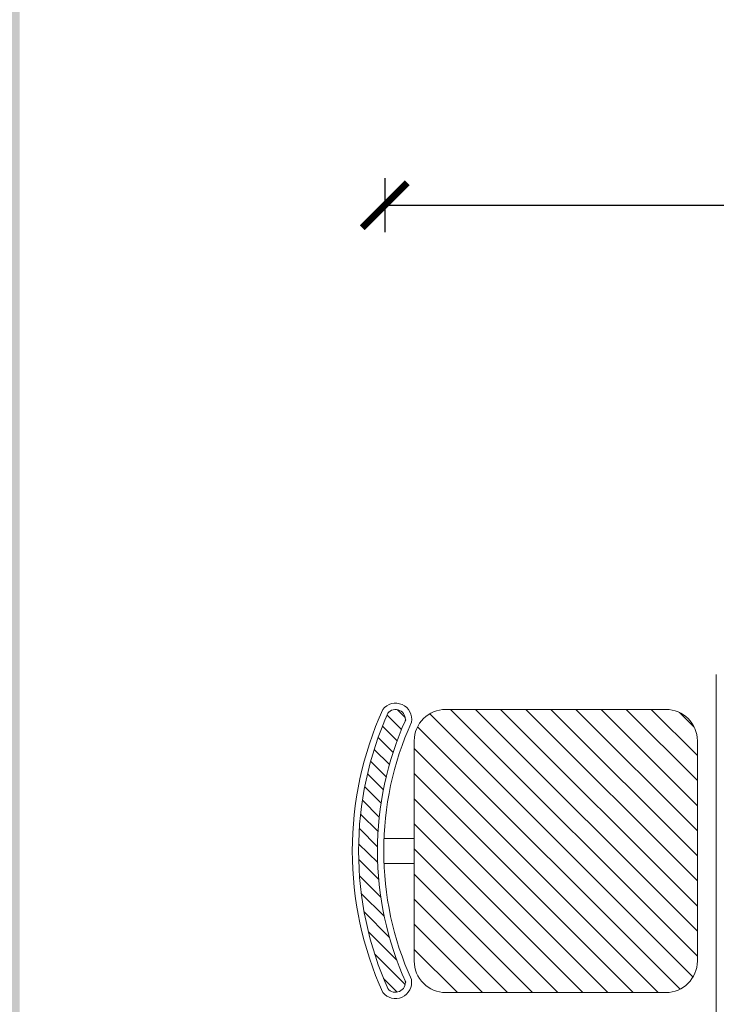
# Model space of a CAD drawing. Units: inches. Extents: x 375 to 1122, y 27 to 1069.
# Tile 115 of 155: x 667 to 705, y 887 to 941. Entities that reach past the tile are written whole.
import ezdxf

# ---------------------------------------------------------------- set-up
doc = ezdxf.new("R2010")
doc.units = ezdxf.units.IN
for name, color, linetype, lineweight in [('A-ANNO-DIMS', 2, 'Continuous', 18), ('A-WALL-PATT', 252, 'Continuous', 13), ('Furniture', 30, 'Continuous', 18)]:
    doc.layers.add(name, color=color, linetype=linetype, lineweight=lineweight)
doc.styles.get("Standard").update_dxf_attribs({"font": 'arial.ttf'})
doc.dimstyles.new('ISO-25', dxfattribs={"dimtxt": 12, "dimasz": 2.5, "dimexe": 1.5, "dimexo": 1.5, "dimtad": 1, "dimdec": 1, "dimlunit": 3, "dimtxsty": 'Standard', "dimblk": 'ARCHTICK', "dimcen": 2.5, "dimadec": 0, "dimazin": 0, "dimtfac": 1, "dimtdec": 1, "dimtmove": 0, "dimatfit": 3, "dimfxl": 1.5, "dimfxlon": 1, "dimarcsym": 0})

# ---------------------------------------------------------------- blocks, each defined once
blk = doc.blocks.new('A$C403C54AD')
for p, q in [((0.8357, 0.5048, -0.0006), (1.9992, 0.5048, -0.0006)), ((1.2329, 0.4785, -0.0006), (0.9275, 0.4785, -0.0006)), ((0.8839, 0.4349, -0.0006), (0.8839, 0.304, -0.0006)), ((1.2765, 0.1295, -0.0006), (1.2765, 0.4349, -0.0006)), ((0.8839, 0.304, -0.0006), (0.8839, 0.1295, -0.0006)), ((0.9275, 0.0859, -0.0006), (1.2329, 0.0859, -0.0006)), ((1.0628, 0.0859, -0.0006), (1.0628, 0.0436, -0.0006)), ((1.0977, 0.0859, -0.0006), (1.0977, 0.0436, -0.0006))]:
    blk.add_line(p, q)
at = {"ltscale": 0.05}
for p, q in [((1.2263, 0.4785, -0.0006), (0.8839, 0.1361, -0.0006)), ((1.1915, 0.4785, -0.0006), (0.8839, 0.1709, -0.0006)), ((1.1567, 0.4785, -0.0006), (0.8839, 0.2057, -0.0006)), ((1.1218, 0.4785, -0.0006), (0.8839, 0.2406, -0.0006)), ((1.087, 0.4785, -0.0006), (0.8839, 0.2754, -0.0006)), ((1.0522, 0.4785, -0.0006), (0.8839, 0.3102, -0.0006)), ((1.0174, 0.4785, -0.0006), (0.8839, 0.3451, -0.0006)), ((0.9825, 0.4785, -0.0006), (0.8839, 0.3799, -0.0006)), ((0.9477, 0.4785, -0.0006), (0.8839, 0.4147, -0.0006)), ((0.9085, 0.4742, -0.0006), (0.8882, 0.4539, -0.0006)), ((1.2551, 0.4725, -0.0006), (0.8899, 0.1073, -0.0006)), ((1.2719, 0.4545, -0.0006), (0.9079, 0.0905, -0.0006)), ((1.2765, 0.4243, -0.0006), (0.9381, 0.0859, -0.0006)), ((1.2765, 0.3895, -0.0006), (0.973, 0.0859, -0.0006)), ((1.2765, 0.3546, -0.0006), (1.0078, 0.0859, -0.0006)), ((1.2765, 0.3198, -0.0006), (1.0426, 0.0859, -0.0006)), ((1.2765, 0.285, -0.0006), (1.0774, 0.0859, -0.0006)), ((1.2765, 0.2501, -0.0006), (1.1123, 0.0859, -0.0006)), ((1.2765, 0.2153, -0.0006), (1.1471, 0.0859, -0.0006)), ((1.2765, 0.1805, -0.0006), (1.1819, 0.0859, -0.0006)), ((1.2765, 0.1457, -0.0006), (1.2168, 0.0859, -0.0006)), ((0.8952, 0.0734, -0.0006), (0.8843, 0.0625, -0.0006)), ((1.2652, 0.0733, -0.0006), (1.2228, 0.0309, -0.0006)), ((0.9118, 0.0682, -0.0006), (0.8918, 0.0483, -0.0006)), ((0.9274, 0.0621, -0.0006), (0.9072, 0.0418, -0.0006)), ((0.9436, 0.0565, -0.0006), (0.923, 0.0359, -0.0006)), ((1.2317, 0.0616, -0.0006), (1.1924, 0.0224, -0.0006)), ((1.276, 0.0624, -0.0006), (1.2569, 0.0433, -0.0006)), ((0.9603, 0.0515, -0.0006), (0.9393, 0.0304, -0.0006)), ((0.9776, 0.047, -0.0006), (0.9561, 0.0255, -0.0006)), ((0.9955, 0.0431, -0.0006), (0.9734, 0.021, -0.0006)), ((1.1708, 0.0443, -0.0006), (1.139, 0.0124, -0.0006)), ((1.1996, 0.0513, -0.0006), (1.1647, 0.0164, -0.0006)), ((1.014, 0.0399, -0.0006), (0.9914, 0.0172, -0.0006)), ((1.0333, 0.0374, -0.0006), (1.0099, 0.014, -0.0006)), ((1.0534, 0.0357, -0.0006), (1.0292, 0.0115, -0.0006)), ((1.0744, 0.0349, -0.0006), (1.0492, 0.0098, -0.0006)), ((1.0964, 0.0352, -0.0006), (1.0701, 0.0088, -0.0006)), ((1.1197, 0.0367, -0.0006), (1.0919, 0.0089, -0.0006)), ((1.1443, 0.0396, -0.0006), (1.1148, 0.01, -0.0006))]:
    blk.add_line(p, q, dxfattribs=at)
for centre, radius, start, end in [((0.9275, 0.4349, -0.0006), 0.0436, 90, 180), ((1.2329, 0.4349, -0.0006), 0.0436, 0, 90), ((0.9275, 0.1295, -0.0006), 0.0436, 180, 270), ((1.2329, 0.1295, -0.0006), 0.0436, 270, 0), ((0.8978, 0.0599, -0.0006), 0.0225, 79.7658, 231.6694), ((1.0802, 0.4774, -0.0006), 0.4338, 245.7176, 294.2824), ((1.2624, 0.0598, -0.0006), 0.0225, 308.8964, 99.6684), ((0.8978, 0.0599, -0.0006), 0.0138, 79.7658, 231.6694), ((1.0802, 0.4774, -0.0006), 0.4425, 245.7176, 294.2824), ((1.2624, 0.0598, -0.0006), 0.0138, 308.8964, 99.6684), ((1.0802, 0.4774, -0.0006), 0.4774, 245.7176, 294.2824), ((1.0802, 0.4774, -0.0006), 0.4687, 245.7176, 294.2824)]:
    blk.add_arc(centre, radius, start, end)
blk = doc.blocks.new('_ArchTick')
at = {"color": 0, "linetype": 'ByBlock', "const_width": 0.15}
blk.add_lwpolyline([(-0.5, -0.5), (0.5, 0.5)], dxfattribs=at)
blk = doc.blocks.new('*D58')
at = {"layer": 'A-ANNO-DIMS', "color": 0, "lineweight": -2, "transparency": 16777216}
for p, q in [((656.912, 835.528), (656.912, 940.287)), ((655.412, 835.528), (658.412, 835.528)), ((656.912, 750.836), (656.912, 835.528)), ((655.412, 750.836), (658.412, 750.836))]:
    blk.add_line(p, q, dxfattribs=at)
at = {"layer": 'Defpoints', "color": 0, "transparency": 16777216}
for p in [(638.071, 835.528), (656.912, 835.528), (638.071, 750.836)]:
    blk.add_point(p, dxfattribs=at)
at = {"layer": 'A-ANNO-DIMS', "color": 0, "lineweight": -2, "transparency": 16777216, "xscale": 2.5, "yscale": 2.5, "zscale": 2.5}
for p, rotation in [((656.912, 835.528), 90), ((656.912, 750.836), 270)]:
    blk.add_blockref('_ArchTick', p, dxfattribs=dict(at, rotation=rotation))
at = {"layer": 'A-ANNO-DIMS', "color": 0, "transparency": 16777216, "insert": (650.082, 889.157), "char_height": 12, "attachment_point": 5, "rotation": 90}
blk.add_mtext('7\'-0 1/2" TYP.', dxfattribs=at)
blk = doc.blocks.new('*D73')
at = {"layer": 'A-ANNO-DIMS', "color": 0, "lineweight": -2, "transparency": 16777216}
for p, q in [((686.757, 932.428), (686.757, 929.428)), ((770.757, 932.428), (770.757, 929.428)), ((686.757, 930.928), (770.757, 930.928)), ((770.757, 930.928), (987.61, 930.928))]:
    blk.add_line(p, q, dxfattribs=at)
at = {"layer": 'Defpoints', "color": 0, "transparency": 16777216}
for p in [(686.757, 943.528), (770.757, 943.528), (770.757, 930.928)]:
    blk.add_point(p, dxfattribs=at)
at = {"layer": 'A-ANNO-DIMS', "color": 0, "lineweight": -2, "transparency": 16777216, "xscale": 2.5, "yscale": 2.5, "zscale": 2.5, "rotation": 180}
blk.add_blockref('_ArchTick', (686.757, 930.928), dxfattribs=at)
at = {"layer": 'A-ANNO-DIMS', "color": 0, "lineweight": -2, "transparency": 16777216, "xscale": 2.5, "yscale": 2.5, "zscale": 2.5}
blk.add_blockref('_ArchTick', (770.757, 930.928), dxfattribs=at)
at = {"layer": 'A-ANNO-DIMS', "color": 0, "transparency": 16777216, "insert": (880.433, 937.757), "char_height": 12, "attachment_point": 5}
blk.add_mtext('2-PANEL SLIDER 7\'-0" TYP.', dxfattribs=at)

msp = doc.modelspace()

# ---------------------------------------------------------------- hatches: boundary and pattern name
at = {"layer": 'A-WALL-PATT'}
h = msp.add_hatch(color=256, dxfattribs=at)
h.dxf.hatch_style = 1
h.paths.add_polyline_path([(962.007, 388.528), (989.007, 388.528), (989.007, 394.528), (962.007, 394.528), (932.007, 394.528), (932.007, 397.528), (923.007, 397.528), (923.007, 394.528), (842.007, 394.528), (842.007, 334.528), (839.507, 334.528), (839.507, 328.528), (854.007, 328.528), (854.007, 334.528), (848.007, 334.528), (848.007, 388.528), (953.007, 388.528), (953.007, 356.081), (962.007, 356.081), (962.007, 358.554), (989.007, 358.554), (989.007, 364.554), (962.007, 364.554)])
h.paths.add_polyline_path([(989.007, 502.528), (932.007, 502.528), (932.007, 583.528), (932.007, 593.528), (923.007, 593.528), (923.007, 583.528), (854.007, 583.528), (854.007, 556.528), (863.007, 556.528), (863.007, 574.528), (923.007, 574.528), (923.007, 502.528), (863.007, 502.528), (863.007, 520.528), (854.007, 520.528), (854.007, 502.528), (773.007, 502.528), (773.007, 493.528), (788.007, 493.528), (788.007, 402.028), (722.007, 402.028), (722.007, 373.528), (728.007, 373.528), (728.007, 396.028), (788.007, 396.028), (788.007, 373.528), (794.007, 373.528), (794.007, 430.528), (814.007, 430.528), (814.007, 436.528), (794.007, 436.528), (794.007, 493.528), (923.007, 493.528), (923.007, 487.528), (932.007, 487.528), (932.007, 493.528), (983.007, 493.528), (983.007, 473.528), (989.007, 473.528)])
h.paths.add_polyline_path([(797.007, 325.528), (805.007, 325.528), (805.007, 328.528), (807.507, 328.528), (807.507, 334.528), (791.007, 334.528), (791.007, 226.528), (770.757, 226.528), (770.757, 217.528), (791.007, 217.528), (791.007, 187.528), (855.007, 187.528), (855.007, 196.528), (797.007, 196.528)])
h.paths.add_polyline_path([(989.007, 238.528), (962.007, 238.528), (962.007, 256.424), (953.007, 256.424), (953.007, 229.528), (980.007, 229.528), (980.007, 196.528), (915.007, 196.528), (915.007, 187.528), (989.007, 187.528)])
h.paths.add_polyline_path([(962.007, 334.528), (884.007, 334.528), (884.007, 328.528), (918.007, 328.528), (918.007, 325.528), (932.007, 325.528), (932.007, 328.528), (953.007, 328.528), (953.007, 304.424), (962.007, 304.424)])
h.paths.add_polyline_path([(606.507, 283.528), (609.507, 283.528), (609.507, 289.528), (600.507, 289.528), (600.507, 196.528), (578.507, 196.528), (578.507, 187.528), (606.507, 187.528), (606.507, 196.528)])
h.paths.add_polyline_path([(666.507, 292.528), (660.507, 292.528), (660.507, 289.528), (633.507, 289.528), (633.507, 283.528), (660.507, 283.528), (660.507, 196.528), (628.007, 196.528), (628.007, 187.528), (630.534, 187.528), (630.534, 160.528), (636.534, 160.528), (636.534, 187.528), (660.507, 187.528), (660.507, 160.528), (666.507, 160.528), (666.507, 217.528), (686.757, 217.528), (686.757, 226.528), (666.507, 226.528)])
h.paths.add_polyline_path([(480.507, 256.424), (471.507, 256.424), (471.507, 238.528), (444.507, 238.528), (444.507, 187.528), (518.507, 187.528), (518.507, 196.528), (453.507, 196.528), (453.507, 229.528), (480.507, 229.528)])
h.paths.add_polyline_path([(480.507, 328.528), (652.507, 328.528), (652.507, 325.528), (660.507, 325.528), (660.507, 322.528), (666.507, 322.528), (666.507, 334.528), (507.507, 334.528), (507.507, 360.528), (498.507, 360.528), (498.507, 334.528), (471.507, 334.528), (471.507, 304.424), (480.507, 304.424)])
h.paths.add_polyline_path([(507.507, 484.528), (498.507, 484.528), (498.507, 444.528), (507.507, 444.528), (507.507, 454.528), (621.507, 454.528), (621.507, 460.528), (507.507, 460.528)])
h.paths.add_polyline_path([(672.507, 604.528), (683.257, 604.528), (683.257, 613.528), (669.507, 613.528), (669.507, 649.528), (663.507, 649.528), (663.507, 589.528), (507.507, 589.528), (507.507, 613.528), (498.507, 613.528), (498.507, 556.528), (507.507, 556.528), (507.507, 580.528), (663.507, 580.528), (663.507, 520.528), (669.507, 520.528), (669.507, 556.528), (683.257, 556.528), (683.257, 565.528), (672.507, 565.528)])
h.paths.add_polyline_path([(731.007, 667.528), (734.007, 667.528), (734.007, 676.528), (728.007, 676.528), (728.007, 715.528), (657.507, 715.528), (657.507, 709.528), (663.507, 709.528), (663.507, 673.528), (669.507, 673.528), (669.507, 709.528), (722.007, 709.528), (722.007, 613.528), (704.757, 613.528), (704.757, 604.528), (722.007, 604.528), (722.007, 565.528), (704.757, 565.528), (704.757, 556.528), (722.007, 556.528), (722.007, 502.528), (722.007, 460.528), (669.507, 460.528), (669.507, 496.528), (663.507, 496.528), (663.507, 460.528), (657.507, 460.528), (657.507, 454.528), (728.007, 454.528), (728.007, 493.528), (734.007, 493.528), (734.007, 502.528), (731.007, 502.528)])
h.paths.add_polyline_path([(986.007, 718.528), (959.007, 718.528), (959.007, 727.528), (950.007, 727.528), (950.007, 709.528), (977.007, 709.528), (977.007, 676.528), (794.007, 676.528), (794.007, 805.528), (802.007, 805.528), (802.007, 808.528), (804.507, 808.528), (804.507, 814.528), (788.007, 814.528), (788.007, 774.028), (728.007, 774.028), (728.007, 796.528), (722.007, 796.528), (722.007, 768.028), (788.007, 768.028), (788.007, 676.528), (773.007, 676.528), (773.007, 667.528), (923.007, 667.528), (923.007, 657.528), (932.007, 657.528), (932.007, 667.528), (986.007, 667.528)])
h.paths.add_polyline_path([(621.507, 715.528), (507.507, 715.528), (507.507, 733.528), (498.507, 733.528), (498.507, 715.528), (498.507, 685.528), (507.507, 685.528), (507.507, 709.528), (621.507, 709.528)])
h.paths.add_polyline_path([(666.507, 847.028), (660.507, 847.028), (660.507, 844.528), (652.507, 844.528), (652.507, 841.528), (480.507, 841.528), (480.507, 859.528), (471.507, 859.528), (471.507, 835.528), (498.507, 835.528), (498.507, 817.528), (507.507, 817.528), (507.507, 835.528), (666.507, 835.528)])
h.paths.add_polyline_path([(480.507, 940.528), (453.507, 940.528), (453.507, 973.528), (518.507, 973.528), (518.507, 982.528), (444.507, 982.528), (444.507, 931.528), (471.507, 931.528), (471.507, 907.528), (480.507, 907.528)])
h.paths.add_polyline_path([(606.507, 982.528), (578.507, 982.528), (578.507, 973.528), (600.507, 973.528), (600.507, 880.528), (609.507, 880.528), (609.507, 886.528), (606.507, 886.528)])
h.paths.add_polyline_path([(666.507, 943.528), (686.757, 943.528), (686.757, 952.528), (666.507, 952.528), (666.507, 1009.528), (660.507, 1009.528), (660.507, 982.528), (636.534, 982.528), (636.534, 1009.528), (630.534, 1009.528), (630.534, 982.528), (628.007, 982.528), (628.007, 973.528), (660.507, 973.528), (660.507, 886.528), (633.507, 886.528), (633.507, 880.528), (660.507, 880.528), (660.507, 877.028), (666.507, 877.028)])
h.paths.add_polyline_path([(986.007, 874.528), (932.007, 874.528), (932.007, 877.528), (923.007, 877.528), (923.007, 874.528), (788.007, 874.528), (788.007, 868.528), (788.007, 844.528), (794.007, 844.528), (794.007, 868.528), (839.007, 868.528), (839.007, 814.528), (836.507, 814.528), (836.507, 808.528), (851.007, 808.528), (851.007, 814.528), (845.007, 814.528), (845.007, 868.528), (986.007, 868.528)])
h.paths.add_polyline_path([(959.007, 838.554), (986.007, 838.554), (986.007, 844.554), (959.007, 844.554), (959.007, 847.028), (950.007, 847.028), (950.007, 814.528), (881.007, 814.528), (881.007, 808.528), (918.007, 808.528), (918.007, 805.528), (932.007, 805.528), (932.007, 808.528), (950.007, 808.528), (950.007, 793.528), (959.007, 793.528)])
h.paths.add_polyline_path([(986.007, 982.528), (899.007, 982.528), (899.007, 973.528), (923.007, 973.528), (923.007, 967.528), (932.007, 967.528), (932.007, 973.528), (980.007, 973.528), (980.007, 953.528), (986.007, 953.528)])
h.paths.add_polyline_path([(851.007, 982.528), (788.007, 982.528), (788.007, 952.528), (770.757, 952.528), (770.757, 943.528), (788.007, 943.528), (788.007, 910.528), (814.007, 910.528), (814.007, 916.528), (794.007, 916.528), (794.007, 973.528), (851.007, 973.528)])

# ---------------------------------------------------------------- block references
at = {"layer": 'Furniture', "xscale": 39.9918517141215, "yscale": 39.9918517141215, "zscale": 39.9918517141215, "rotation": 270}
msp.add_blockref('A$C403C54AD', (684.955, 938.316, 0.024), dxfattribs=at)

# ---------------------------------------------------------------- dimensions: what is measured, and where the dimension line sits
at = {"layer": 'A-ANNO-DIMS'}
dim = msp.add_linear_dim(base=(770.757, 930.928), p1=(686.757, 943.528), p2=(770.757, 943.528), text='2-PANEL SLIDER <> TYP.', dimstyle='ISO-25', override={"dimdec": 1, "dimlfac": 1, "dimrnd": 0, "dimzin": 1, "dimdsep": 46, "dimlunit": 4, "dimfrac": 2}, dxfattribs=at)
dim.commit()
dim.dimension.update_dxf_attribs({"geometry": '*D73', "text_midpoint": (880.433, 937.757)})
dim = msp.add_linear_dim(base=(656.912, 835.528), p1=(638.071, 750.836), p2=(638.071, 835.528), angle=90, text='<> TYP.', dimstyle='ISO-25', override={"dimdec": 1, "dimlfac": 1, "dimrnd": 0, "dimzin": 1, "dimdsep": 46, "dimlunit": 4, "dimfrac": 2}, dxfattribs=at)
dim.commit()
dim.dimension.update_dxf_attribs({"geometry": '*D58', "text_midpoint": (650.082, 889.157)})

doc.saveas('drawing.dxf')
